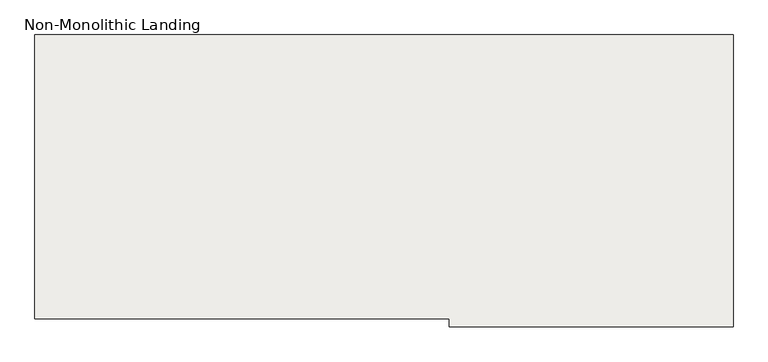
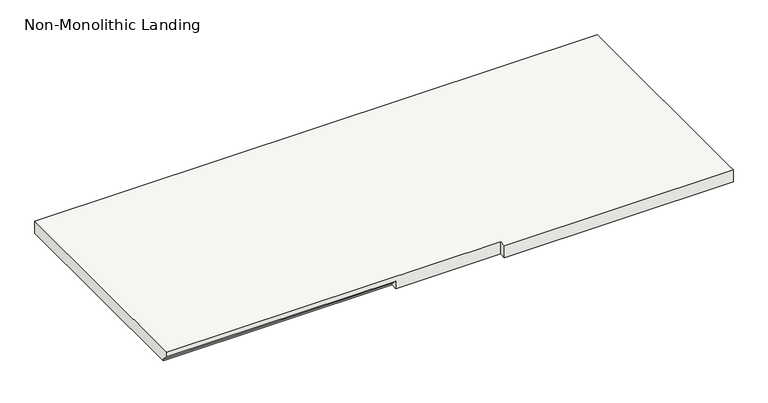
"""IFC4 building model written with IfcOpenShell, lengths in millimetres: slab geometry, Non-Monolithic Landing."""

from ifc_helpers import new_model, si_unit, origin, place, context, project, spatial, faceted_brep, source, transform, mapped, element, save


def non_monolithic_landing_cf1353f8(model_context):
    return source(origin(), model_context, "Body", "Brep", [
        faceted_brep([(131.9501403, 2113.4257925, 2012.95), (131.9501403, 2138.8257925, 1987.55), (1046.3501403, 2138.8257925, 1987.55), (1046.3501403, 2113.4257925, 2012.95), (1465.4501403, 2113.4257925, 2032.0), (1465.4501403, 2088.0257925, 2032.0), (2379.8501403, 2088.0257925, 2032.0), (2379.8501403, 2113.4257925, 2032.0), (2379.8501403, 3027.8257925, 2032.0), (131.9501403, 3027.8257925, 2032.0), (131.9501403, 2113.4257925, 2032.0), (1046.3501403, 2138.8257925, 1981.2), (131.9501403, 2138.8257925, 1981.2), (131.9501403, 3027.8257925, 1981.2), (2379.8501403, 3027.8257925, 1981.2), (2379.8501403, 2113.4257925, 1981.2), (2379.8501403, 2088.0257925, 1981.2), (1465.4501403, 2088.0257925, 1981.2), (1465.4501403, 2113.4257925, 1981.2), (1046.3501403, 2113.4257925, 1981.2)], [[[0, 1, 2, 3]], [[4, 5, 6, 7, 8, 9, 10]], [[11, 12, 13, 14, 15, 16, 17, 18, 19]], [[12, 11, 2, 1]], [[11, 19, 3, 2]], [[4, 10, 0, 3, 19, 18]], [[5, 4, 18, 17]], [[6, 5, 17, 16]], [[7, 6, 16, 15]], [[8, 7, 15, 14]], [[9, 8, 14, 13]], [[10, 9, 13, 12, 1, 0]]]),
    ])


if __name__ == "__main__":
    model = new_model("IFC4")
    model_context = context("Model", 3, world=origin())
    ifc_project = project(units=[si_unit("LENGTHUNIT", "METRE", prefix="MILLI")], contexts=[model_context])
    site = spatial("IfcSite", under=ifc_project)
    building = spatial("IfcBuilding", under=site)
    placement = place(None, origin())
    non_monolithic_landing_shape = non_monolithic_landing_cf1353f8(model_context)
    element("IfcSlab", 1, ObjectType="Non-Monolithic Landing", at=placement, inside=building, context=model_context, shape_type="MappedRepresentation", body=[
        mapped(non_monolithic_landing_shape, transform((0.0, 0.0, 0.0), x_axis=(1.0, 0.0, 0.0), y_axis=(0.0, 1.0, 0.0), z_axis=(0.0, 0.0, 1.0))),
    ])
    save(model, "model.ifc")
